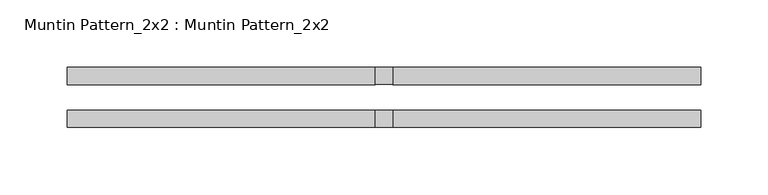
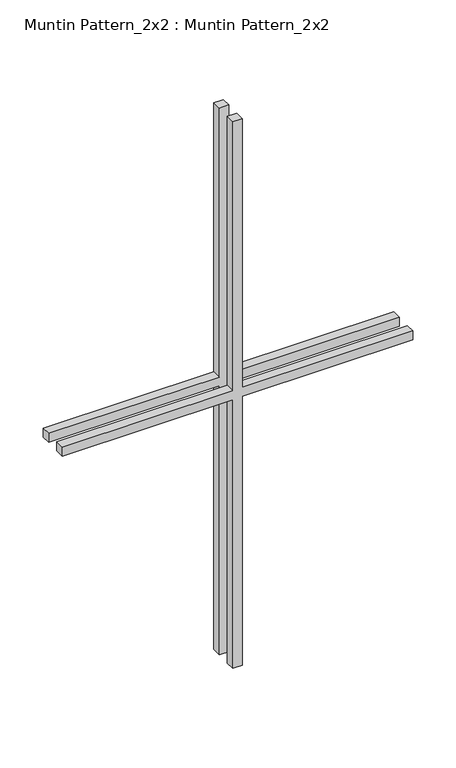
"""IFC4 building model written with IfcOpenShell, lengths in millimetres: proxy geometry, Muntin Pattern_2x2 : Muntin Pattern_2x2."""

from ifc_helpers import new_model, si_unit, frame, origin, place, context, project, spatial, polyline, outline, extrude, source, transform, mapped, element, save


def muntin_pattern_2x2_muntin_pattern_2x2_49143b38(model_context):
    return source(origin(), model_context, "Body", "SweptSolid", [
        extrude(outline(polyline([(393.7, -6.35), (393.7, -234.95), (381.0, -234.95), (381.0, -6.35), (0.0, -6.35), (0.0, 6.35), (381.0, 6.35), (381.0, 234.95), (393.7, 234.95), (393.7, 6.35), (774.7, 6.35), (774.7, -6.35), (393.7, -6.35)])), frame((0.0, -22.225, 0.0), z_axis=(0.0, 1.0, 0.0), x_axis=(0.0, 0.0, 1.0)), (0.0, 0.0, 1.0), 12.7),
        extrude(outline(polyline([(393.7, -6.35), (393.7, -234.95), (381.0, -234.95), (381.0, -6.35), (0.0, -6.35), (0.0, 6.35), (381.0, 6.35), (381.0, 234.95), (393.7, 234.95), (393.7, 6.35), (774.7, 6.35), (774.7, -6.35), (393.7, -6.35)])), frame((0.0, 9.525, 0.0), z_axis=(0.0, 1.0, 0.0), x_axis=(0.0, 0.0, 1.0)), (0.0, 0.0, 1.0), 12.7),
    ])


if __name__ == "__main__":
    model = new_model("IFC4")
    model_context = context("Model", 3, world=origin())
    ifc_project = project(units=[si_unit("LENGTHUNIT", "METRE", prefix="MILLI")], contexts=[model_context])
    site = spatial("IfcSite", under=ifc_project)
    building = spatial("IfcBuilding", under=site)
    placement = place(None, origin())
    muntin_pattern_2x2_muntin_pattern_2x2_shape = muntin_pattern_2x2_muntin_pattern_2x2_49143b38(model_context)
    element("IfcBuildingElementProxy", 1, Name="Muntin Pattern_2x2 : Muntin Pattern_2x2", ObjectType="Muntin Pattern_2x2 : Muntin Pattern_2x2", at=placement, inside=building, context=model_context, shape_type="MappedRepresentation", body=[
        mapped(muntin_pattern_2x2_muntin_pattern_2x2_shape, transform((0.0, 0.0, 0.0), x_axis=(1.0, 0.0, 0.0), y_axis=(0.0, 1.0, 0.0), z_axis=(0.0, 0.0, 1.0))),
    ])
    save(model, "model.ifc")

# Revit data of these elements
# Type "Muntin Pattern_2x2 : Muntin Pattern_2x2"
#   Width [instance default] = 4' - 0"
#   Thickness = 0' - 0 1/2"
#   Height [instance default] = 4' - 0"
#   Distance = 0' - 0 3/4"
#   Interior Material [instance default] = none
#   Exterior Material [instance default] = none
#   Default Elevation = 0
# Element 1 (IfcBuildingElementProxy, "Muntin Pattern_2x2 : Muntin Pattern_2x2")
#   Width = 1' - 6 1/2"
#   Height = 2' - 6 1/2"
#   Interior Material = Wood - Stained
#   Exterior Material = Clad - White
#   Materials on its faces: "Clad - White", "Wood - Stained"
# Materials
#   "Clad - White": class "Wood", colour RGB 242 242 238, transparency 0, Cost = 0
#   "Wood - Stained": class "Wood", colour RGB 224 178 126, transparency 0, Cost = 0
